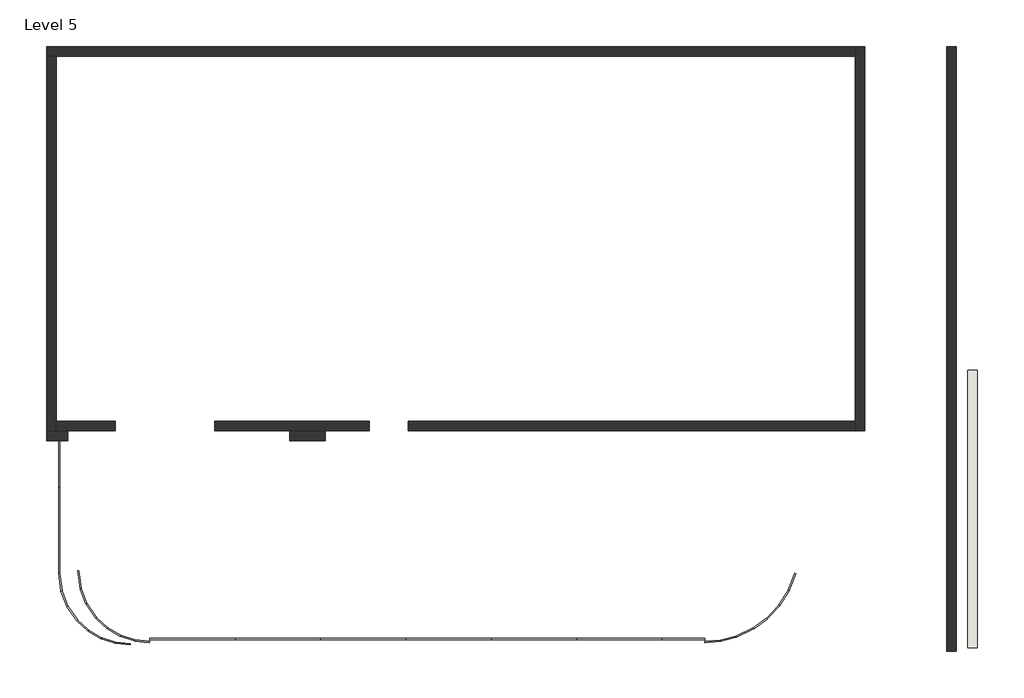
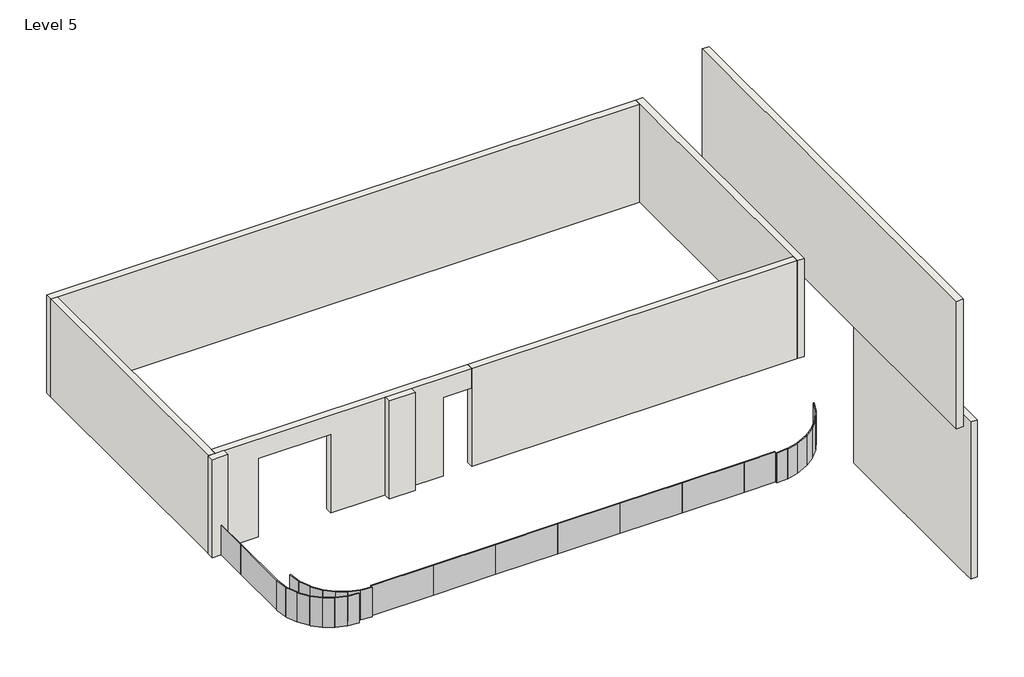
# One storey, incomplete: 30 plates, 9 walls.
"""IFC4 building model written with IfcOpenShell, lengths in millimetres."""

from ifc_helpers import new_model, si_unit, frame, origin, place, context, project, spatial, polyline, outline, extrude, faceted_brep, transform, mapped, element, save
from components import system_panel_glazed_95be5de7, system_panel_glazed_8746fe8c, system_panel_glazed_70ef586e, system_panel_glazed_2e848b93, system_panel_glazed_d6f392a9, system_panel_glazed_76d2efde, system_panel_glazed_97d0a6f3, system_panel_glazed_abbe3f8f, system_panel_glazed_0a91d840, system_panel_glazed_0f72cd4c, system_panel_glazed_404bb2e9, system_panel_glazed_ab35909a, system_panel_glazed_299ce7ab

model = new_model("IFC4")

# Units and contexts
model_context = context("Model", 3, world=origin())
ifc_project = project(units=[si_unit("LENGTHUNIT", "METRE", prefix="MILLI")], contexts=[model_context])

# Site, building, storey
site = spatial("IfcSite", under=ifc_project)
building = spatial("IfcBuilding", under=site)
storey = spatial("IfcBuildingStorey", under=building, Name="Level 5", Elevation=12192.0)

# Plates
placement = place(None, origin())
system_panel_glazed_shape = system_panel_glazed_95be5de7(model_context)
element("IfcPlate", 1, ObjectType="System Panel : Glazed", at=placement, inside=storey, context=model_context, shape_type="MappedRepresentation", body=[
    mapped(system_panel_glazed_shape, transform((-15410.278953, 2109.2432662, 11893.55), x_axis=(0.0, 1.0, 0.0), y_axis=(-1.0, 0.0, 0.0), z_axis=(0.0, 0.0, 1.0))),
])
system_panel_glazed_2_shape = system_panel_glazed_8746fe8c(model_context)
element("IfcPlate", 2, ObjectType="System Panel : Glazed", at=placement, inside=storey, context=model_context, shape_type="MappedRepresentation", body=[
    mapped(system_panel_glazed_2_shape, transform((-15386.0907484, 1006.1948552, 11893.55), x_axis=(-0.12717730440498629, 0.9918799994174101, 0.0), y_axis=(-0.9918799994174101, -0.12717730440498629, 0.0), z_axis=(0.0, 0.0, 1.0))),
])
element("IfcPlate", 3, ObjectType="System Panel : Glazed", at=placement, inside=storey, context=model_context, shape_type="MappedRepresentation", body=[
    mapped(system_panel_glazed_2_shape, transform((-14975.5447019, 1056.9948552, 11906.25), x_axis=(-0.12717730440498623, 0.9918799994174101, 0.0), y_axis=(-0.9918799994174101, -0.12717730440498623, 0.0), z_axis=(0.0, 0.0, 1.0))),
])
system_panel_glazed_3_shape = system_panel_glazed_70ef586e(model_context)
element("IfcPlate", 4, ObjectType="System Panel : Glazed", at=placement, inside=storey, context=model_context, shape_type="MappedRepresentation", body=[
    mapped(system_panel_glazed_3_shape, transform((-15300.9211317, 659.6162823, 11893.55), x_axis=(-0.36020879862792127, 0.9328717068230925, 0.0), y_axis=(-0.9328717068230925, -0.36020879862792127, 0.0), z_axis=(0.0, 0.0, 1.0))),
])
element("IfcPlate", 5, ObjectType="System Panel : Glazed", at=placement, inside=storey, context=model_context, shape_type="MappedRepresentation", body=[
    mapped(system_panel_glazed_3_shape, transform((-14890.3750853, 710.4162823, 11906.25), x_axis=(-0.36020879862792143, 0.9328717068230924, 0.0), y_axis=(-0.9328717068230924, -0.36020879862792143, 0.0), z_axis=(0.0, 0.0, 1.0))),
])
system_panel_glazed_4_shape = system_panel_glazed_2e848b93(model_context)
element("IfcPlate", 6, ObjectType="System Panel : Glazed", at=placement, inside=storey, context=model_context, shape_type="MappedRepresentation", body=[
    mapped(system_panel_glazed_4_shape, transform((-15136.4134084, 351.6891221, 11893.55), x_axis=(-0.5680307758785693, 0.8230073132450225, 0.0), y_axis=(-0.8230073132450225, -0.5680307758785693, 0.0), z_axis=(0.0, 0.0, 1.0))),
])
element("IfcPlate", 7, ObjectType="System Panel : Glazed", at=placement, inside=storey, context=model_context, shape_type="MappedRepresentation", body=[
    mapped(system_panel_glazed_4_shape, transform((-14725.8673619, 402.4891221, 11906.25), x_axis=(-0.5680307758785693, 0.8230073132450225, 0.0), y_axis=(-0.8230073132450225, -0.5680307758785693, 0.0), z_axis=(0.0, 0.0, 1.0))),
])
system_panel_glazed_5_shape = system_panel_glazed_d6f392a9(model_context)
element("IfcPlate", 8, ObjectType="System Panel : Glazed", at=placement, inside=storey, context=model_context, shape_type="MappedRepresentation", body=[
    mapped(system_panel_glazed_5_shape, transform((-14917.4266334, 96.3103352, 11893.55), x_axis=(-0.7386085467399861, 0.6741345671916296, 0.0), y_axis=(-0.6741345671916296, -0.7386085467399861, 0.0), z_axis=(0.0, 0.0, 1.0))),
])
element("IfcPlate", 9, ObjectType="System Panel : Glazed", at=placement, inside=storey, context=model_context, shape_type="MappedRepresentation", body=[
    mapped(system_panel_glazed_5_shape, transform((-14506.880587, 147.1103352, 11906.25), x_axis=(-0.7386085467399861, 0.6741345671916296, 0.0), y_axis=(-0.6741345671916296, -0.7386085467399861, 0.0), z_axis=(0.0, 0.0, 1.0))),
])
system_panel_glazed_6_shape = system_panel_glazed_76d2efde(model_context)
element("IfcPlate", 10, ObjectType="System Panel : Glazed", at=placement, inside=storey, context=model_context, shape_type="MappedRepresentation", body=[
    mapped(system_panel_glazed_6_shape, transform((-14071.8974005, -283.9578788, 11893.55), x_axis=(-0.994403599652405, 0.10564791052519545, 0.0), y_axis=(-0.10564791052519545, -0.994403599652405, 0.0), z_axis=(0.0, 0.0, 1.0))),
])
element("IfcPlate", 11, ObjectType="System Panel : Glazed", at=placement, inside=storey, context=model_context, shape_type="MappedRepresentation", body=[
    mapped(system_panel_glazed_6_shape, transform((-14665.5846616, -88.8381812, 11893.55), x_axis=(-0.8631975005225224, 0.5048663933078434, 0.0), y_axis=(-0.5048663933078434, -0.8631975005225224, 0.0), z_axis=(0.0, 0.0, 1.0))),
])
element("IfcPlate", 12, ObjectType="System Panel : Glazed", at=placement, inside=storey, context=model_context, shape_type="MappedRepresentation", body=[
    mapped(system_panel_glazed_6_shape, transform((-14379.1060319, -217.9354353, 11893.55), x_axis=(-0.9500075321236097, 0.31222698299219553, 0.0), y_axis=(-0.31222698299219553, -0.9500075321236097, 0.0), z_axis=(0.0, 0.0, 1.0))),
])
element("IfcPlate", 13, ObjectType="System Panel : Glazed", at=placement, inside=storey, context=model_context, shape_type="MappedRepresentation", body=[
    mapped(system_panel_glazed_6_shape, transform((-13661.3513541, -233.1578788, 11906.25), x_axis=(-0.994403599652405, 0.10564791052519545, 0.0), y_axis=(-0.10564791052519545, -0.994403599652405, 0.0), z_axis=(0.0, 0.0, 1.0))),
])
element("IfcPlate", 14, ObjectType="System Panel : Glazed", at=placement, inside=storey, context=model_context, shape_type="MappedRepresentation", body=[
    mapped(system_panel_glazed_6_shape, transform((-14255.0386151, -38.0381812, 11906.25), x_axis=(-0.8631975005225224, 0.5048663933078434, 0.0), y_axis=(-0.5048663933078434, -0.8631975005225224, 0.0), z_axis=(0.0, 0.0, 1.0))),
])
element("IfcPlate", 15, ObjectType="System Panel : Glazed", at=placement, inside=storey, context=model_context, shape_type="MappedRepresentation", body=[
    mapped(system_panel_glazed_6_shape, transform((-13968.5599855, -167.1354353, 11906.25), x_axis=(-0.9500075321236097, 0.31222698299219553, 0.0), y_axis=(-0.31222698299219553, -0.9500075321236097, 0.0), z_axis=(0.0, 0.0, 1.0))),
])
system_panel_glazed_7_shape = system_panel_glazed_97d0a6f3(model_context)
element("IfcPlate", 16, ObjectType="System Panel : Glazed", at=placement, inside=storey, context=model_context, shape_type="MappedRepresentation", body=[
    mapped(system_panel_glazed_7_shape, transform((-15410.278953, 3525.3612705, 11893.55), x_axis=(0.0, 1.0, 0.0), y_axis=(-1.0, 0.0, 0.0), z_axis=(0.0, 0.0, 1.0))),
])
system_panel_glazed_8_shape = system_panel_glazed_abbe3f8f(model_context)
element("IfcPlate", 17, ObjectType="System Panel : Glazed", at=placement, inside=storey, context=model_context, shape_type="MappedRepresentation", body=[
    mapped(system_panel_glazed_8_shape, transform((-12589.8398441, -249.8497962, 11899.9), x_axis=(1.0, 0.0, 0.0), y_axis=(0.0, 1.0, 0.0), z_axis=(0.0, 0.0, 1.0))),
])
element("IfcPlate", 18, ObjectType="System Panel : Glazed", at=placement, inside=storey, context=model_context, shape_type="MappedRepresentation", body=[
    mapped(system_panel_glazed_8_shape, transform((-10761.0398441, -249.8497962, 11899.9), x_axis=(1.0, 0.0, 0.0), y_axis=(0.0, 1.0, 0.0), z_axis=(0.0, 0.0, 1.0))),
])
element("IfcPlate", 19, ObjectType="System Panel : Glazed", at=placement, inside=storey, context=model_context, shape_type="MappedRepresentation", body=[
    mapped(system_panel_glazed_8_shape, transform((-8932.2398441, -249.8497962, 11899.9), x_axis=(1.0, 0.0, 0.0), y_axis=(0.0, 1.0, 0.0), z_axis=(0.0, 0.0, 1.0))),
])
element("IfcPlate", 20, ObjectType="System Panel : Glazed", at=placement, inside=storey, context=model_context, shape_type="MappedRepresentation", body=[
    mapped(system_panel_glazed_8_shape, transform((-7103.4398441, -249.8497962, 11899.9), x_axis=(1.0, 0.0, 0.0), y_axis=(0.0, 1.0, 0.0), z_axis=(0.0, 0.0, 1.0))),
])
element("IfcPlate", 21, ObjectType="System Panel : Glazed", at=placement, inside=storey, context=model_context, shape_type="MappedRepresentation", body=[
    mapped(system_panel_glazed_8_shape, transform((-5274.6398441, -249.8497962, 11899.9), x_axis=(1.0, 0.0, 0.0), y_axis=(0.0, 1.0, 0.0), z_axis=(0.0, 0.0, 1.0))),
])
element("IfcPlate", 22, ObjectType="System Panel : Glazed", at=placement, inside=storey, context=model_context, shape_type="MappedRepresentation", body=[
    mapped(system_panel_glazed_8_shape, transform((-3445.8398441, -249.8497962, 11899.9), x_axis=(1.0, 0.0, 0.0), y_axis=(0.0, 1.0, 0.0), z_axis=(0.0, 0.0, 1.0))),
])
system_panel_glazed_9_shape = system_panel_glazed_0a91d840(model_context)
element("IfcPlate", 23, ObjectType="System Panel : Glazed", at=placement, inside=storey, context=model_context, shape_type="MappedRepresentation", body=[
    mapped(system_panel_glazed_9_shape, transform((-2074.2398441, -249.8497962, 11899.9), x_axis=(1.0, 0.0, 0.0), y_axis=(0.0, 1.0, 0.0), z_axis=(0.0, 0.0, 1.0))),
])
system_panel_glazed_10_shape = system_panel_glazed_0f72cd4c(model_context)
element("IfcPlate", 24, ObjectType="System Panel : Glazed", at=placement, inside=storey, context=model_context, shape_type="MappedRepresentation", body=[
    mapped(system_panel_glazed_10_shape, transform((-771.4163948, -48.7697426, 11899.9), x_axis=(-0.9036899876908312, -0.42818734935463165, 0.0), y_axis=(0.42818734935463165, -0.9036899876908312, 0.0), z_axis=(0.0, 0.0, 1.0))),
])
system_panel_glazed_11_shape = system_panel_glazed_404bb2e9(model_context)
element("IfcPlate", 25, ObjectType="System Panel : Glazed", at=placement, inside=storey, context=model_context, shape_type="MappedRepresentation", body=[
    mapped(system_panel_glazed_11_shape, transform((-444.4490728, 142.6972628, 11899.9), x_axis=(-0.8053846593635025, -0.5927525204180369, 0.0), y_axis=(0.5927525204180369, -0.8053846593635025, 0.0), z_axis=(0.0, 0.0, 1.0))),
])
system_panel_glazed_12_shape = system_panel_glazed_ab35909a(model_context)
element("IfcPlate", 26, ObjectType="System Panel : Glazed", at=placement, inside=storey, context=model_context, shape_type="MappedRepresentation", body=[
    mapped(system_panel_glazed_12_shape, transform((224.8474052, 1018.3780736, 11899.9), x_axis=(-0.36299643103623197, -0.931790529601454, 0.0), y_axis=(0.931790529601454, -0.36299643103623197, 0.0), z_axis=(0.0, 0.0, 1.0))),
])
element("IfcPlate", 27, ObjectType="System Panel : Glazed", at=placement, inside=storey, context=model_context, shape_type="MappedRepresentation", body=[
    mapped(system_panel_glazed_12_shape, transform((-175.4793802, 383.396855, 11899.9), x_axis=(-0.6842264553506641, -0.7292696057002963, 0.0), y_axis=(0.7292696057002963, -0.6842264553506641, 0.0), z_axis=(0.0, 0.0, 1.0))),
])
element("IfcPlate", 28, ObjectType="System Panel : Glazed", at=placement, inside=storey, context=model_context, shape_type="MappedRepresentation", body=[
    mapped(system_panel_glazed_12_shape, transform((55.1017493, 681.7104644, 11899.9), x_axis=(-0.53331287683458, -0.8459180666012662, 0.0), y_axis=(0.8459180666012662, -0.53331287683458, 0.0), z_axis=(0.0, 0.0, 1.0))),
])
system_panel_glazed_13_shape = system_panel_glazed_299ce7ab(model_context)
element("IfcPlate", 29, ObjectType="System Panel : Glazed", at=placement, inside=storey, context=model_context, shape_type="MappedRepresentation", body=[
    mapped(system_panel_glazed_13_shape, transform((-1121.1318098, -179.6234093, 11899.9), x_axis=(-0.968084530428735, -0.2506239053733217, 0.0), y_axis=(0.2506239053733217, -0.968084530428735, 0.0), z_axis=(0.0, 0.0, 1.0))),
])
element("IfcPlate", 30, ObjectType="System Panel : Glazed", at=placement, inside=storey, context=model_context, shape_type="MappedRepresentation", body=[
    mapped(system_panel_glazed_13_shape, transform((-1450.1543246, -235.7241331, 11899.9), x_axis=(-0.9964369295237279, -0.08434124424814608, 0.0), y_axis=(0.08434124424814608, -0.9964369295237279, 0.0), z_axis=(0.0, 0.0, 1.0))),
])

# Walls
element("IfcWall", 31, ObjectType="Generic - 8\" brown", at=placement, inside=storey, context=model_context, shape_type="SweptSolid", body=[
    extrude(outline(polyline([(-15255.3533244, 4027.0792748), (-15712.5533244, 4027.0792748), (-15712.5533244, 4230.2792748), (-15255.3533244, 4230.2792748), (-15255.3533244, 4027.0792748)])), frame((0.0, 0.0, 11893.55), z_axis=(0.0, 0.0, 1.0), x_axis=(1.0, 0.0, 0.0)), (0.0, 0.0, 1.0), 3048.0),
])
element("IfcWall", 32, ObjectType="Generic - 8\" brown", at=placement, inside=storey, context=model_context, shape_type="SweptSolid", body=[
    extrude(outline(polyline([(-9743.5533244, 4027.0792748), (-10505.5533244, 4027.0792748), (-10505.5533244, 4230.2792748), (-9743.5533244, 4230.2792748), (-9743.5533244, 4027.0792748)])), frame((0.0, 0.0, 11893.55), z_axis=(0.0, 0.0, 1.0), x_axis=(1.0, 0.0, 0.0)), (0.0, 0.0, 1.0), 3048.0),
])
element("IfcWall", 33, ObjectType="Generic - 8\" white wood", at=placement, inside=storey, context=model_context, shape_type="Brep", body=[
    faceted_brep([(4226.4466756, -405.3567338, 7013.3940217), (4226.4466756, 5538.2432662, 7013.3940217), (4226.4466756, 5538.2432662, 11890.209914), (4226.4466756, -405.3567338, 11890.209914), (4023.2466756, -405.3567338, 7013.3940217), (4023.2466756, -405.3567338, 11890.209914), (4023.2466756, 5538.2432662, 11890.209914), (4023.2466756, 5538.2432662, 7013.3940217), (4023.2466756, 3042.8292748, 7013.3940217), (4023.2466756, 2903.1292748, 7013.3940217), (4023.2466756, 2814.2292748, 7013.3940217), (4023.2466756, 2674.5292748, 7013.3940217), (4023.2466756, 2585.6292748, 7013.3940217), (4023.2466756, 2445.9292748, 7013.3940217), (4023.2466756, 2382.4292748, 7013.3940217), (4023.2466756, 2242.7292748, 7013.3940217), (4023.2466756, 2179.2292748, 7013.3940217), (4023.2466756, 2039.5292748, 7013.3940217), (4023.2466756, 1950.6292748, 7013.3940217), (4023.2466756, 1810.9292748, 7013.3940217), (4023.2466756, 1722.0292748, 7013.3940217), (4023.2466756, 1582.3292748, 7013.3940217), (4023.2466756, 1518.8292748, 7013.3940217), (4023.2466756, 1379.1292748, 7013.3940217), (4023.2466756, 1315.6292748, 7013.3940217), (4023.2466756, 1175.9292748, 7013.3940217), (4023.2466756, 1112.4292748, 7013.3940217), (4023.2466756, 972.7292748, 7013.3940217), (4023.2466756, 909.2292748, 7013.3940217), (4023.2466756, 769.5292748, 7013.3940217), (4023.2466756, 706.0292748, 7013.3940217), (4023.2466756, 566.3292748, 7013.3940217), (4023.2466756, 502.8292748, 7013.3940217), (4023.2466756, 363.1292748, 7013.3940217), (4023.2466756, 299.6292748, 7013.3940217), (4023.2466756, 159.9292748, 7013.3940217), (4023.2466756, 96.4292748, 7013.3940217), (4023.2466756, -43.2707252, 7013.3940217), (4023.2466756, -106.7707252, 7013.3940217), (4023.2466756, -246.4707252, 7013.3940217), (4023.2466756, -309.9707252, 7013.3940217), (4048.6466756, -405.3567338, 7013.3940217)], [[[0, 1, 2, 3]], [[4, 5, 6, 7, 8, 9, 10, 11, 12, 13, 14, 15, 16, 17, 18, 19, 20, 21, 22, 23, 24, 25, 26, 27, 28, 29, 30, 31, 32, 33, 34, 35, 36, 37, 38, 39, 40]], [[1, 0, 41, 4, 40, 39, 38, 37, 36, 35, 34, 33, 32, 31, 30, 29, 28, 27, 26, 25, 24, 23, 22, 21, 20, 19, 18, 17, 16, 15, 14, 13, 12, 11, 10, 9, 8, 7]], [[2, 1, 7, 6]], [[3, 2, 6, 5]], [[0, 3, 5, 4, 41]]]),
])
element("IfcWall", 34, ObjectType="Generic - 8\" wood", at=placement, inside=storey, context=model_context, shape_type="Brep", body=[
    faceted_brep([(-15712.5533244, 12269.3792748, 11893.55), (-15509.3533244, 12269.3792748, 11893.55), (1610.2466756, 12269.3792748, 11893.55), (1610.2466756, 12269.3792748, 14941.55), (-15509.3533244, 12269.3792748, 14941.55), (-15712.5533244, 12269.3792748, 14941.55), (-15712.5533244, 12472.5792748, 11893.55), (-15712.5533244, 12472.5792748, 14941.55), (1610.2466756, 12472.5792748, 14941.55), (1610.2466756, 12472.5792748, 11893.55)], [[[0, 1, 2, 3, 4, 5]], [[6, 7, 8, 9]], [[2, 1, 0, 6, 9]], [[5, 4, 3, 8, 7]], [[0, 5, 7, 6]], [[3, 2, 9, 8]]]),
])
element("IfcWall", 35, ObjectType="Generic - 8\" wood", at=placement, inside=storey, context=model_context, shape_type="Brep", body=[
    faceted_brep([(-15509.3533244, 4242.9792748, 11893.55), (-15509.3533244, 4446.1792748, 11893.55), (-15509.3533244, 12269.3792748, 11893.55), (-15509.3533244, 12269.3792748, 14941.55), (-15509.3533244, 4446.1792748, 14941.55), (-15509.3533244, 4242.9792748, 14941.55), (-15712.5533244, 4242.9792748, 11893.55), (-15712.5533244, 4242.9792748, 14941.55), (-15712.5533244, 12269.3792748, 14941.55), (-15712.5533244, 12269.3792748, 11893.55)], [[[0, 1, 2, 3, 4, 5]], [[6, 7, 8, 9]], [[2, 1, 0, 6, 9]], [[5, 4, 3, 8, 7]], [[0, 5, 7, 6]], [[3, 2, 9, 8]]]),
])
element("IfcWall", 36, ObjectType="Generic - 8\" wood", at=placement, inside=storey, context=model_context, shape_type="Brep", body=[
    faceted_brep([(1610.2466756, 12472.5792748, 11893.55), (1610.2466756, 12269.3792748, 11893.55), (1610.2466756, 4446.1792748, 11893.55), (1610.2466756, 4242.9792748, 11893.55), (1610.2466756, 4242.9792748, 14941.55), (1610.2466756, 4446.1792748, 14941.55), (1610.2466756, 12269.3792748, 14941.55), (1610.2466756, 12472.5792748, 14941.55), (1813.4466756, 12472.5792748, 11893.55), (1813.4466756, 12472.5792748, 14941.55), (1813.4466756, 4242.9792748, 14941.55), (1813.4466756, 4242.9792748, 11893.55)], [[[0, 1, 2, 3, 4, 5, 6, 7]], [[8, 9, 10, 11]], [[3, 2, 1, 0, 8, 11]], [[7, 6, 5, 4, 10, 9]], [[0, 7, 9, 8]], [[4, 3, 11, 10]]]),
])
element("IfcWall", 37, ObjectType="Generic - 8\" wood", at=placement, inside=storey, context=model_context, shape_type="SweptSolid", body=[
    extrude(outline(polyline([(11893.55, -15509.3533244), (11893.55, -14243.2931037), (14331.95, -14243.2931037), (14331.95, -12109.6931037), (11893.55, -12109.6931037), (11893.55, -8802.0384076), (14331.95, -8802.0384076), (14331.95, -7965.5533244), (14941.55, -7965.5533244), (14941.55, -15509.3533244), (11893.55, -15509.3533244)])), frame((0.0, 4242.9792748, 0.0), z_axis=(0.0, 1.0, 0.0), x_axis=(0.0, 0.0, 1.0)), (0.0, 0.0, 1.0), 203.2),
])
element("IfcWall", 38, ObjectType="Generic - 8\" wood", at=placement, inside=storey, context=model_context, shape_type="SweptSolid", body=[
    extrude(outline(polyline([(3566.0466756, -481.4207252), (3566.0466756, 12472.5792748), (3769.2466756, 12472.5792748), (3769.2466756, -481.4207252), (3566.0466756, -481.4207252)])), frame((0.0, 0.0, 11887.2), z_axis=(0.0, 0.0, 1.0), x_axis=(1.0, 0.0, 0.0)), (0.0, 0.0, 1.0), 3968.75),
])
element("IfcWall", 39, ObjectType="Generic - 8\" wood 2", at=placement, inside=storey, context=model_context, shape_type="SweptSolid", body=[
    extrude(outline(polyline([(-7965.5533244, 4446.1792748), (1610.2466756, 4446.1792748), (1610.2466756, 4242.9792748), (-7965.5533244, 4242.9792748), (-7965.5533244, 4446.1792748)])), frame((0.0, 0.0, 11893.55), z_axis=(0.0, 0.0, 1.0), x_axis=(1.0, 0.0, 0.0)), (0.0, 0.0, 1.0), 3048.0),
])

save(model, "model.ifc")

# Revit data of these elements
# Type "System Panel : Glazed"
#   Construction Type Id = "GSP4R"
#   Analytic Construction = "1/8 in Pilkington single glazing"
#   Visual Light Transmittance = 0.9
#   Solar Heat Gain Coefficient = 0.86
#   Heat Transfer Coefficient (U) = 1.18115 BTU/(h·ft²·°F)
# Type "Generic - 8\" brown"
#   Assembly Code = "B2010"
#   Layers, outside or top first: 0' - 8" "Door - Panel" (function 1)
# Type "Generic - 8\" white wood"
#   Assembly Code = "B2010"
#   Layers, outside or top first: 0' - 8" "Tile, Porcelain, 4in" (function 1)
# Type "Generic - 8\" wood"
#   Assembly Code = "B2010"
#   Layers, outside or top first: 0' - 8" "Cherry" (function 1)
# Type "Generic - 8\" wood 2"
#   Assembly Code = "B2010"
#   Layers, outside or top first: 0' - 8" "Concrete, Precast" (function 1)
# Elements 1, 2, 3, 4, 5, 6, 7, 8, 9, 10, 11, 12, 13, 14, 15, 16, 17, 18, 19, 20, 21, 22, 23, 24, 25, 26, 27, 28, 29, 30 (IfcPlate, "System Panel : Glazed")
#   Phase Created = New Construction
#   Materials on its faces: "Glass"
# Elements 31, 32 (IfcWall, "Generic - 8\" brown")
#   built-in parameter 1001111 = -0' - 11 3/4"
#   Top Offset = 0' - 0"
#   Base Offset = -0' - 11 3/4"
#   Unconnected Height = 10' - 0"
#   wall height = 10' - 0"
#   Phase Created = New Construction
#   Base Constraint = Level 5
#   Materials on its faces: "Door - Panel"
# Element 33 (IfcWall, "Generic - 8\" white wood")
#   built-in parameter 1001111 = -16' - 11.88213"
#   Top Offset = 0' - 0"
#   Base Offset = -16' - 11.88213"
#   Unconnected Height = 16' - 0.00063"
#   wall height = 16' - 0.00063"
#   Phase Created = New Construction
#   Base Constraint = Level 5
#   Materials on its faces: "Tile, Porcelain, 4in"
# Elements 34, 35, 37 (IfcWall, "Generic - 8\" wood")
#   built-in parameter 1001111 = -0' - 11 3/4"
#   Top Offset = 0' - 0"
#   Base Offset = -0' - 11 3/4"
#   Unconnected Height = 10' - 0"
#   wall height = 10' - 0"
#   Phase Created = New Construction
#   Base Constraint = Level 5
#   Materials on its faces: "Cherry"
# Element 36 (IfcWall, "Generic - 8\" wood")
#   built-in parameter 1001111 = -0' - 11 3/4"
#   Top Offset = 0' - 0"
#   Base Offset = -0' - 11 3/4"
#   Unconnected Height = 10' - 0"
#   wall height = 10' - 0"
#   Phase Created = New Construction
#   Base Constraint = Level 5
#   Materials on its faces: "Cherry", "Concrete, Precast"
# Element 38 (IfcWall, "Generic - 8\" wood")
#   built-in parameter 1001111 = -1' - 0"
#   Top Offset = 0' - 0"
#   Base Offset = -1' - 0"
#   Unconnected Height = 13' - 0 1/4"
#   wall height = 13' - 0 1/4"
#   Phase Created = New Construction
#   Base Constraint = Level 5
#   Materials on its faces: "Cherry"
# Element 39 (IfcWall, "Generic - 8\" wood 2")
#   built-in parameter 1001111 = -0' - 11 3/4"
#   Top Offset = 0' - 0"
#   Base Offset = -0' - 11 3/4"
#   Unconnected Height = 10' - 0"
#   wall height = 10' - 0"
#   Phase Created = New Construction
#   Base Constraint = Level 5
#   Materials on its faces: "Concrete, Precast"
# Materials
#   "Door - Panel": class "Wood", colour RGB 210 159 95, transparency 0, Cost = 0
#   "Tile, Porcelain, 4in": class "Generic", colour RGB 89 87 158, transparency 0, Description = "Porcelain tile, 4\", white", Cost = 0
#   "Cherry": class "Wood", colour RGB 238 208 179, transparency 0, Description = "Prunus Serotina", Cost = 0
#   "Concrete, Precast": class "Concrete", colour RGB 198 187 187, transparency 0, Description = "Precast concrete", Cost = 0
#   "Glass": class "Glass", colour RGB 0 128 192, transparency 0.75, Description = "Soda Lime Glass", Cost = 0
